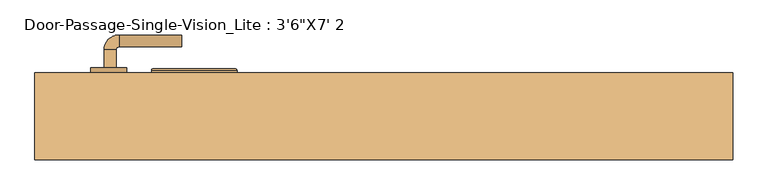
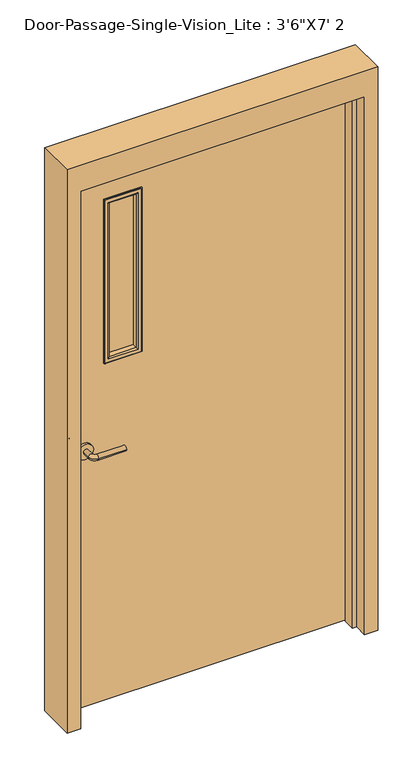
"""IFC4 building model written with IfcOpenShell, lengths in millimetres: door geometry."""

from ifc_helpers import new_model, si_unit, point, frame, frame_2d, origin, place, context, project, spatial, polyline, circle_curve, ellipse_curve, trimmed, segment, composite_curve, outline, extrude, faceted_brep, source, transform, mapped, element, save
from ifc_brep_helpers import plane_surface, cylinder_surface, revolved_surface, advanced_brep


def door_586e558e(model_context):
    return source(origin(), model_context, "Body", "SolidModel", [
        advanced_brep(
        [(-468.390625, 42.8, 1016.0), (-448.390625, 42.8, 1016.0), (-448.390625, 12.8, 1016.0), (-468.390625, 12.8, 1016.0), (-443.390625, 7.8, 1016.0), (-443.390625, -12.2, 1016.0), (-338.390625, -12.2, 1016.0), (-338.390625, 7.8, 1016.0)],
        [
            (0, 1, circle_curve(frame((-458.390625, 42.8, 1016.0), z_axis=(0.0, 1.0, 0.0), x_axis=(1.0, 0.0, 0.0)), 10.0)),
            (1, 0, circle_curve(frame((-458.390625, 42.8, 1016.0), z_axis=(0.0, 1.0, 0.0), x_axis=(1.0, 0.0, 0.0)), 10.0)),
            (1, 2),
            (2, 3, circle_curve(frame((-458.390625, 12.8, 1016.0), z_axis=(0.0, 1.0, 0.0), x_axis=(1.0, 0.0, 0.0)), 10.0)),
            (3, 0),
            (3, 2, circle_curve(frame((-458.390625, 12.8, 1016.0), z_axis=(0.0, 1.0, 0.0), x_axis=(1.0, 0.0, 0.0)), 10.0)),
            (4, 5, circle_curve(frame((-443.390625, -2.2, 1016.0), z_axis=(-1.0, 0.0, 0.0), x_axis=(0.0, 1.0, 0.0)), 10.0)),
            (5, 3, circle_curve(frame((-443.390625, 12.8, 1016.0), z_axis=(0.0, 0.0, -1.0), x_axis=(-1.0, 0.0, 0.0)), 25.0)),
            (2, 4, circle_curve(frame((-443.390625, 12.8, 1016.0), z_axis=(0.0, 0.0, 1.0), x_axis=(-1.0, 0.0, 0.0)), 5.0)),
            (5, 4, circle_curve(frame((-443.390625, -2.2, 1016.0), z_axis=(-1.0, 0.0, 0.0), x_axis=(0.0, 1.0, 0.0)), 10.0)),
            (6, 7, circle_curve(frame((-338.390625, -2.2, 1016.0), z_axis=(1.0, 0.0, 0.0), x_axis=(0.0, 1.0, 0.0)), 10.0)),
            (7, 6, circle_curve(frame((-338.390625, -2.2, 1016.0), z_axis=(1.0, 0.0, 0.0), x_axis=(0.0, 1.0, 0.0)), 10.0)),
            (4, 7),
            (6, 5),
        ],
        [
            plane_surface(frame((-458.390625, 42.8, 1016.0), z_axis=(0.0, 1.0, 0.0), x_axis=(0.0, 0.0, 1.0))),
            cylinder_surface(frame((-458.390625, 42.8, 1016.0), z_axis=(0.0, 1.0, 0.0), x_axis=(1.0, 0.0, 0.0)), 10.0),
            revolved_surface(trimmed(ellipse_curve(frame((-458.390625, 12.8, 1016.0), z_axis=(0.0, -1.0, 0.0), x_axis=(1.0, 0.0, 0.0)), 10.0, 10.0), [point((-468.390625, 12.8, 1016.0))], [point((-448.390625, 12.8, 1016.0))], True, "CARTESIAN"), (-443.390625, 12.8, 1016.0), (0.0, 0.0, -1.0)),
            revolved_surface(trimmed(ellipse_curve(frame((-458.390625, 12.8, 1016.0), z_axis=(0.0, -1.0, 0.0), x_axis=(1.0, 0.0, 0.0)), 10.0, 10.0), [point((-448.390625, 12.8, 1016.0))], [point((-468.390625, 12.8, 1016.0))], True, "CARTESIAN"), (-443.390625, 12.8, 1016.0), (0.0, 0.0, -1.0)),
            plane_surface(frame((-338.390625, -2.2, 1016.0), z_axis=(1.0, 0.0, 0.0), x_axis=(0.0, 0.0, 1.0))),
            cylinder_surface(frame((-443.390625, -2.2, 1016.0), z_axis=(-1.0, 0.0, 0.0), x_axis=(0.0, 1.0, 0.0)), 10.0),
        ],
        [
            (0, [[1, 2]]),
            (1, [[3, 4, 5, -2]]),
            (1, [[-5, 6, -3, -1]]),
            (2, [[7, 8, -4, 9]]),
            (3, [[10, -9, -6, -8]]),
            (4, [[11, 12]]),
            (5, [[13, -11, 14, -7]]),
            (5, [[-14, -12, -13, -10]]),
        ],
    ),
        extrude(outline(composite_curve([segment(trimmed(circle_curve(frame_2d((1016.0, -460.890625)), 30.0), [point((1016.0, -490.890625))], [point((1016.0, -430.890625))], False, "CARTESIAN"), True, "CONTINUOUS"), segment(trimmed(circle_curve(frame_2d((1016.0, -460.890625)), 30.0), [point((1016.0, -430.890625))], [point((1016.0, -490.890625))], False, "CARTESIAN"), True, "CONTINUOUS")], self_intersect=False)), frame((0.0, 42.8, 0.0), z_axis=(0.0, 1.0, 0.0), x_axis=(0.0, 0.0, 1.0)), (0.0, 0.0, 1.0), 8.0),
        advanced_brep(
        [(-468.390625, 103.25, 1016.0), (-448.390625, 103.25, 1016.0), (-468.390625, 133.25, 1016.0), (-448.390625, 133.25, 1016.0), (-443.390625, 138.25, 1016.0), (-443.390625, 158.25, 1016.0), (-338.390625, 158.25, 1016.0), (-338.390625, 138.25, 1016.0)],
        [
            (0, 1, circle_curve(frame((-458.390625, 103.25, 1016.0), z_axis=(0.0, -1.0, 0.0), x_axis=(1.0, 0.0, 0.0)), 10.0)),
            (1, 0, circle_curve(frame((-458.390625, 103.25, 1016.0), z_axis=(0.0, -1.0, 0.0), x_axis=(1.0, 0.0, 0.0)), 10.0)),
            (0, 2),
            (2, 3, circle_curve(frame((-458.390625, 133.25, 1016.0), z_axis=(0.0, -1.0, 0.0), x_axis=(1.0, 0.0, 0.0)), 10.0)),
            (3, 1),
            (3, 2, circle_curve(frame((-458.390625, 133.25, 1016.0), z_axis=(0.0, -1.0, 0.0), x_axis=(1.0, 0.0, 0.0)), 10.0)),
            (4, 3, circle_curve(frame((-443.390625, 133.25, 1016.0), z_axis=(0.0, 0.0, 1.0), x_axis=(-1.0, 0.0, 0.0)), 5.0)),
            (2, 5, circle_curve(frame((-443.390625, 133.25, 1016.0), z_axis=(0.0, 0.0, -1.0), x_axis=(-1.0, 0.0, 0.0)), 25.0)),
            (5, 4, circle_curve(frame((-443.390625, 148.25, 1016.0), z_axis=(-1.0, 0.0, 0.0), x_axis=(0.0, -1.0, 0.0)), 10.0)),
            (4, 5, circle_curve(frame((-443.390625, 148.25, 1016.0), z_axis=(-1.0, 0.0, 0.0), x_axis=(0.0, -1.0, 0.0)), 10.0)),
            (6, 7, circle_curve(frame((-338.390625, 148.25, 1016.0), z_axis=(1.0, 0.0, 0.0), x_axis=(0.0, -1.0, 0.0)), 10.0)),
            (7, 6, circle_curve(frame((-338.390625, 148.25, 1016.0), z_axis=(1.0, 0.0, 0.0), x_axis=(0.0, -1.0, 0.0)), 10.0)),
            (5, 6),
            (7, 4),
        ],
        [
            plane_surface(frame((-458.390625, 103.25, 1016.0), z_axis=(0.0, -1.0, 0.0), x_axis=(0.0, 0.0, 1.0))),
            cylinder_surface(frame((-458.390625, 103.25, 1016.0), z_axis=(0.0, -1.0, 0.0), x_axis=(1.0, 0.0, 0.0)), 10.0),
            revolved_surface(trimmed(ellipse_curve(frame((-458.390625, 133.25, 1016.0), z_axis=(0.0, -1.0, 0.0), x_axis=(1.0, 0.0, 0.0)), 10.0, 10.0), [point((-468.390625, 133.25, 1016.0))], [point((-448.390625, 133.25, 1016.0))], True, "CARTESIAN"), (-443.390625, 133.25, 1016.0), (0.0, 0.0, -1.0)),
            revolved_surface(trimmed(ellipse_curve(frame((-458.390625, 133.25, 1016.0), z_axis=(0.0, -1.0, 0.0), x_axis=(1.0, 0.0, 0.0)), 10.0, 10.0), [point((-448.390625, 133.25, 1016.0))], [point((-468.390625, 133.25, 1016.0))], True, "CARTESIAN"), (-443.390625, 133.25, 1016.0), (0.0, 0.0, -1.0)),
            plane_surface(frame((-338.390625, 148.25, 1016.0), z_axis=(1.0, 0.0, 0.0), x_axis=(0.0, 0.0, 1.0))),
            cylinder_surface(frame((-443.390625, 148.25, 1016.0), z_axis=(-1.0, 0.0, 0.0), x_axis=(0.0, -1.0, 0.0)), 10.0),
        ],
        [
            (0, [[1, 2]]),
            (1, [[-1, 3, 4, 5]]),
            (1, [[-2, -5, 6, -3]]),
            (2, [[7, -4, 8, 9]]),
            (3, [[-8, -6, -7, 10]]),
            (4, [[11, 12]]),
            (5, [[-9, 13, -12, 14]]),
            (5, [[-10, -14, -11, -13]]),
        ],
    ),
        extrude(outline(composite_curve([segment(trimmed(circle_curve(frame_2d((1016.0, -460.890625)), 30.0), [point((1016.0, -490.890625))], [point((1016.0, -430.890625))], False, "CARTESIAN"), True, "CONTINUOUS"), segment(trimmed(circle_curve(frame_2d((1016.0, -460.890625)), 30.0), [point((1016.0, -430.890625))], [point((1016.0, -490.890625))], False, "CARTESIAN"), True, "CONTINUOUS")], self_intersect=False)), frame((0.0, 95.25, 0.0), z_axis=(0.0, 1.0, 0.0), x_axis=(0.0, 0.0, 1.0)), (0.0, 0.0, 1.0), 8.0),
        extrude(outline(polyline([(2133.6, -533.4), (0.0, -533.4), (0.0, 533.4), (2133.6, 533.4), (2133.6, -533.4)]), holes=[polyline([(1981.2, -381.0), (1981.2, -254.0), (1346.2, -254.0), (1346.2, -381.0), (1981.2, -381.0)])]), frame((0.0, 50.8, 0.0), z_axis=(0.0, 1.0, 0.0), x_axis=(0.0, 0.0, 1.0)), (0.0, 0.0, 1.0), 44.45),
        faceted_brep([(533.4, 46.0375, 0.0), (533.4, 95.25, 0.0), (584.2, 95.25, 0.0), (584.2, -50.8, 0.0), (533.4, -50.8, 0.0), (533.4, -1.5875, 0.0), (517.525, -1.5875, 0.0), (517.525, 46.0375, 0.0), (533.4, 46.0375, 2133.6), (533.4, 95.25, 2133.6), (-533.4, 95.25, 2133.6), (-533.4, 95.25, 0.0), (-584.2, 95.25, 0.0), (-584.2, 95.25, 2235.2), (584.2, 95.25, 2235.2), (584.2, -50.8, 2235.2), (-584.2, -50.8, 2235.2), (-584.2, -50.8, 0.0), (-533.4, -50.8, 0.0), (-533.4, -50.8, 2133.6), (533.4, -50.8, 2133.6), (533.4, -1.5875, 2133.6), (-533.4, -1.5875, 2133.6), (-533.4, -1.5875, 0.0), (-517.525, -1.5875, 0.0), (-517.525, -1.5875, 2117.725), (517.525, -1.5875, 2117.725), (517.525, 46.0375, 2117.725), (-517.525, 46.0375, 2117.725), (-517.525, 46.0375, 0.0), (-533.4, 46.0375, 0.0), (-533.4, 46.0375, 2133.6)], [[[0, 1, 2, 3, 4, 5, 6, 7]], [[1, 0, 8, 9]], [[2, 1, 9, 10, 11, 12, 13, 14]], [[3, 2, 14, 15]], [[4, 3, 15, 16, 17, 18, 19, 20]], [[5, 4, 20, 21]], [[6, 5, 21, 22, 23, 24, 25, 26]], [[7, 6, 26, 27]], [[0, 7, 27, 28, 29, 30, 31, 8]], [[9, 8, 31, 10]], [[20, 19, 22, 21]], [[26, 25, 28, 27]], [[12, 11, 30, 29, 24, 23, 18, 17]], [[11, 10, 31, 30]], [[13, 12, 17, 16]], [[19, 18, 23, 22]], [[25, 24, 29, 28]], [[15, 14, 13, 16]]]),
        extrude(outline(polyline([(-254.0, 69.85), (-381.0, 69.85), (-381.0, 76.2), (-254.0, 76.2), (-254.0, 69.85)])), frame((0.0, 0.0, 1346.2), z_axis=(0.0, 0.0, 1.0), x_axis=(1.0, 0.0, 0.0)), (0.0, 0.0, 1.0), 635.0),
        advanced_brep(
        [(-381.0, 76.2, 1981.2), (-381.0, 95.25, 1981.2), (-381.0, 95.25, 1346.2), (-381.0, 76.2, 1346.2), (-369.0, 96.25, 1969.2), (-369.0, 76.2, 1969.2), (-369.0, 76.2, 1358.2), (-369.0, 96.25, 1358.2), (-374.0, 101.25, 1974.2), (-374.0, 101.25, 1353.2), (-389.0, 99.25, 1989.2), (-387.0, 101.25, 1987.2), (-387.0, 101.25, 1340.2), (-389.0, 99.25, 1338.2), (-389.0, 95.25, 1989.2), (-389.0, 95.25, 1338.2), (-254.0, 95.25, 1346.2), (-254.0, 76.2, 1346.2), (-266.0, 76.2, 1358.2), (-266.0, 96.25, 1358.2), (-261.0, 101.25, 1353.2), (-248.0, 101.25, 1340.2), (-246.0, 99.25, 1338.2), (-246.0, 95.25, 1338.2), (-254.0, 95.25, 1981.2), (-254.0, 76.2, 1981.2), (-266.0, 76.2, 1969.2), (-266.0, 96.25, 1969.2), (-261.0, 101.25, 1974.2), (-248.0, 101.25, 1987.2), (-246.0, 99.25, 1989.2), (-246.0, 95.25, 1989.2)],
        [
            (0, 1),
            (1, 2),
            (2, 3),
            (3, 0),
            (4, 5),
            (5, 6),
            (6, 7),
            (7, 4),
            (8, 4, ellipse_curve(frame((-374.0, 96.25, 1974.2), z_axis=(-0.7071067811865475, 0.0, -0.7071067811865475), x_axis=(-0.7071067811865474, 0.0, 0.7071067811865476)), 7.0710678, 5.0)),
            (7, 9, ellipse_curve(frame((-374.0, 96.25, 1353.2), z_axis=(-0.7071067811865475, 0.0, 0.7071067811865475), x_axis=(0.7071067811865474, 0.0, 0.7071067811865476)), 7.0710678, 5.0)),
            (9, 8),
            (10, 11, ellipse_curve(frame((-387.0, 99.25, 1987.2), z_axis=(-0.7071067811865475, 0.0, -0.7071067811865475), x_axis=(-0.7071067811865474, 0.0, 0.7071067811865476)), 2.8284271, 2.0)),
            (11, 12),
            (12, 13, ellipse_curve(frame((-387.0, 99.25, 1340.2), z_axis=(-0.7071067811865475, 0.0, 0.7071067811865475), x_axis=(0.7071067811865474, 0.0, 0.7071067811865476)), 2.8284271, 2.0)),
            (13, 10),
            (14, 10),
            (13, 15),
            (15, 14),
            (2, 16),
            (16, 17),
            (17, 3),
            (6, 18),
            (18, 19),
            (19, 7),
            (19, 20, ellipse_curve(frame((-261.0, 96.25, 1353.2), z_axis=(-0.7071067811865475, 0.0, -0.7071067811865475), x_axis=(-0.7071067811865476, 0.0, 0.7071067811865474)), 7.0710678, 5.0)),
            (20, 9),
            (12, 21),
            (21, 22, ellipse_curve(frame((-248.0, 99.25, 1340.2), z_axis=(-0.7071067811865475, 0.0, -0.7071067811865475), x_axis=(-0.7071067811865476, 0.0, 0.7071067811865474)), 2.8284271, 2.0)),
            (22, 13),
            (22, 23),
            (23, 15),
            (16, 24),
            (24, 25),
            (25, 17),
            (18, 26),
            (26, 27),
            (27, 19),
            (27, 28, ellipse_curve(frame((-261.0, 96.25, 1974.2), z_axis=(0.7071067811865475, 0.0, -0.7071067811865475), x_axis=(-0.7071067811865474, 0.0, -0.7071067811865476)), 7.0710678, 5.0)),
            (28, 20),
            (21, 29),
            (29, 30, ellipse_curve(frame((-248.0, 99.25, 1987.2), z_axis=(0.7071067811865475, 0.0, -0.7071067811865475), x_axis=(-0.7071067811865474, 0.0, -0.7071067811865476)), 2.8284271, 2.0)),
            (30, 22),
            (30, 31),
            (31, 23),
            (31, 14),
            (1, 24),
            (0, 25),
            (5, 26),
            (4, 27),
            (8, 28),
            (11, 29),
            (10, 30),
        ],
        [
            plane_surface(frame((-381.0, 95.25, 1981.2), z_axis=(-1.0, 0.0, 0.0), x_axis=(0.0, 0.0, -1.0))),
            plane_surface(frame((-369.0, 76.2, 1969.2), z_axis=(1.0, 0.0, 0.0), x_axis=(0.0, 0.0, -1.0))),
            cylinder_surface(frame((-374.0, 96.25, 1981.2), z_axis=(0.0, 0.0, 1.0), x_axis=(-1.0, 0.0, 0.0)), 5.0),
            cylinder_surface(frame((-387.0, 99.25, 1981.2), z_axis=(0.0, 0.0, 1.0), x_axis=(-1.0, 0.0, 0.0)), 2.0),
            plane_surface(frame((-389.0, 99.25, 1989.2), z_axis=(-1.0, 0.0, 0.0), x_axis=(0.0, 0.0, -1.0))),
            plane_surface(frame((-381.0, 95.25, 1346.2), z_axis=(0.0, 0.0, -1.0), x_axis=(1.0, 0.0, 0.0))),
            plane_surface(frame((-369.0, 76.2, 1358.2), z_axis=(0.0, 0.0, 1.0), x_axis=(1.0, 0.0, 0.0))),
            cylinder_surface(frame((-381.0, 96.25, 1353.2), z_axis=(-1.0, 0.0, 0.0), x_axis=(0.0, 0.0, -1.0)), 5.0),
            cylinder_surface(frame((-381.0, 99.25, 1340.2), z_axis=(-1.0, 0.0, 0.0), x_axis=(0.0, 0.0, -1.0)), 2.0),
            plane_surface(frame((-389.0, 99.25, 1338.2), z_axis=(0.0, 0.0, -1.0), x_axis=(1.0, 0.0, 0.0))),
            plane_surface(frame((-254.0, 95.25, 1346.2), z_axis=(1.0, 0.0, 0.0), x_axis=(0.0, 0.0, 1.0))),
            plane_surface(frame((-266.0, 76.2, 1358.2), z_axis=(-1.0, 0.0, 0.0), x_axis=(0.0, 0.0, 1.0))),
            cylinder_surface(frame((-261.0, 96.25, 1346.2), z_axis=(0.0, 0.0, -1.0), x_axis=(1.0, 0.0, 0.0)), 5.0),
            cylinder_surface(frame((-248.0, 99.25, 1346.2), z_axis=(0.0, 0.0, -1.0), x_axis=(1.0, 0.0, 0.0)), 2.0),
            plane_surface(frame((-246.0, 99.25, 1338.2), z_axis=(1.0, 0.0, 0.0), x_axis=(0.0, 0.0, 1.0))),
            plane_surface(frame((-246.0, 95.25, 1989.2), z_axis=(0.0, -1.0, 0.0), x_axis=(-1.0, 0.0, 0.0))),
            plane_surface(frame((-254.0, 95.25, 1981.2), z_axis=(0.0, 0.0, 1.0), x_axis=(-1.0, 0.0, 0.0))),
            plane_surface(frame((-254.0, 76.2, 1981.2), z_axis=(0.0, -1.0, 0.0), x_axis=(-1.0, 0.0, 0.0))),
            plane_surface(frame((-266.0, 76.2, 1969.2), z_axis=(0.0, 0.0, -1.0), x_axis=(-1.0, 0.0, 0.0))),
            cylinder_surface(frame((-254.0, 96.25, 1974.2), z_axis=(1.0, 0.0, 0.0), x_axis=(0.0, 0.0, 1.0)), 5.0),
            plane_surface(frame((-261.0, 101.25, 1974.2), z_axis=(0.0, 1.0, 0.0), x_axis=(-1.0, 0.0, 0.0))),
            cylinder_surface(frame((-254.0, 99.25, 1987.2), z_axis=(1.0, 0.0, 0.0), x_axis=(0.0, 0.0, 1.0)), 2.0),
            plane_surface(frame((-246.0, 99.25, 1989.2), z_axis=(0.0, 0.0, 1.0), x_axis=(-1.0, 0.0, 0.0))),
        ],
        [
            (0, [[1, 2, 3, 4]]),
            (1, [[5, 6, 7, 8]]),
            (2, [[9, -8, 10, 11]]),
            (3, [[12, 13, 14, 15]]),
            (4, [[16, -15, 17, 18]]),
            (5, [[-3, 19, 20, 21]]),
            (6, [[-7, 22, 23, 24]]),
            (7, [[-10, -24, 25, 26]]),
            (8, [[-14, 27, 28, 29]]),
            (9, [[-17, -29, 30, 31]]),
            (10, [[-20, 32, 33, 34]]),
            (11, [[-23, 35, 36, 37]]),
            (12, [[-25, -37, 38, 39]]),
            (13, [[-28, 40, 41, 42]]),
            (14, [[-30, -42, 43, 44]]),
            (15, [[-31, -44, 45, -18], [46, -32, -19, -2]]),
            (16, [[-33, -46, -1, 47]]),
            (17, [[-21, -34, -47, -4], [48, -35, -22, -6]]),
            (18, [[-36, -48, -5, 49]]),
            (19, [[-38, -49, -9, 50]]),
            (20, [[51, -40, -27, -13], [-26, -39, -50, -11]]),
            (21, [[-41, -51, -12, 52]]),
            (22, [[-43, -52, -16, -45]]),
        ],
    ),
        advanced_brep(
        [(-381.0, 69.85, 1346.2), (-381.0, 50.8, 1346.2), (-381.0, 50.8, 1981.2), (-381.0, 69.85, 1981.2), (-369.0, 49.8, 1358.2), (-369.0, 69.85, 1358.2), (-369.0, 69.85, 1969.2), (-369.0, 49.8, 1969.2), (-374.0, 44.8, 1353.2), (-374.0, 44.8, 1974.2), (-389.0, 46.8, 1338.2), (-387.0, 44.8, 1340.2), (-387.0, 44.8, 1987.2), (-389.0, 46.8, 1989.2), (-389.0, 50.8, 1338.2), (-389.0, 50.8, 1989.2), (-254.0, 50.8, 1981.2), (-254.0, 69.85, 1981.2), (-266.0, 69.85, 1969.2), (-266.0, 49.8, 1969.2), (-261.0, 44.8, 1974.2), (-248.0, 44.8, 1987.2), (-246.0, 46.8, 1989.2), (-246.0, 50.8, 1989.2), (-254.0, 50.8, 1346.2), (-254.0, 69.85, 1346.2), (-266.0, 69.85, 1358.2), (-266.0, 49.8, 1358.2), (-261.0, 44.8, 1353.2), (-248.0, 44.8, 1340.2), (-246.0, 46.8, 1338.2), (-246.0, 50.8, 1338.2)],
        [
            (0, 1),
            (1, 2),
            (2, 3),
            (3, 0),
            (4, 5),
            (5, 6),
            (6, 7),
            (7, 4),
            (8, 4, ellipse_curve(frame((-374.0, 49.8, 1353.2), z_axis=(-0.7071067811865475, 0.0, 0.7071067811865475), x_axis=(-0.7071067811865474, 0.0, -0.7071067811865476)), 7.0710678, 5.0)),
            (7, 9, ellipse_curve(frame((-374.0, 49.8, 1974.2), z_axis=(-0.7071067811865475, 0.0, -0.7071067811865475), x_axis=(0.7071067811865474, 0.0, -0.7071067811865476)), 7.0710678, 5.0)),
            (9, 8),
            (10, 11, ellipse_curve(frame((-387.0, 46.8, 1340.2), z_axis=(-0.7071067811865475, 0.0, 0.7071067811865475), x_axis=(-0.7071067811865474, 0.0, -0.7071067811865476)), 2.8284271, 2.0)),
            (11, 12),
            (12, 13, ellipse_curve(frame((-387.0, 46.8, 1987.2), z_axis=(-0.7071067811865475, 0.0, -0.7071067811865475), x_axis=(0.7071067811865474, 0.0, -0.7071067811865476)), 2.8284271, 2.0)),
            (13, 10),
            (14, 10),
            (13, 15),
            (15, 14),
            (2, 16),
            (16, 17),
            (17, 3),
            (6, 18),
            (18, 19),
            (19, 7),
            (19, 20, ellipse_curve(frame((-261.0, 49.8, 1974.2), z_axis=(-0.7071067811865475, 0.0, 0.7071067811865475), x_axis=(-0.7071067811865476, 0.0, -0.7071067811865474)), 7.0710678, 5.0)),
            (20, 9),
            (12, 21),
            (21, 22, ellipse_curve(frame((-248.0, 46.8, 1987.2), z_axis=(-0.7071067811865475, 0.0, 0.7071067811865475), x_axis=(-0.7071067811865476, 0.0, -0.7071067811865474)), 2.8284271, 2.0)),
            (22, 13),
            (22, 23),
            (23, 15),
            (16, 24),
            (24, 25),
            (25, 17),
            (18, 26),
            (26, 27),
            (27, 19),
            (27, 28, ellipse_curve(frame((-261.0, 49.8, 1353.2), z_axis=(0.7071067811865475, 0.0, 0.7071067811865475), x_axis=(-0.7071067811865474, 0.0, 0.7071067811865476)), 7.0710678, 5.0)),
            (28, 20),
            (21, 29),
            (29, 30, ellipse_curve(frame((-248.0, 46.8, 1340.2), z_axis=(0.7071067811865475, 0.0, 0.7071067811865475), x_axis=(-0.7071067811865474, 0.0, 0.7071067811865476)), 2.8284271, 2.0)),
            (30, 22),
            (30, 31),
            (31, 23),
            (31, 14),
            (1, 24),
            (0, 25),
            (5, 26),
            (4, 27),
            (8, 28),
            (11, 29),
            (10, 30),
        ],
        [
            plane_surface(frame((-381.0, 50.8, 1346.2), z_axis=(-1.0, 0.0, 0.0), x_axis=(0.0, 0.0, 1.0))),
            plane_surface(frame((-369.0, 69.85, 1358.2), z_axis=(1.0, 0.0, 0.0), x_axis=(0.0, 0.0, 1.0))),
            cylinder_surface(frame((-374.0, 49.8, 1346.2), z_axis=(0.0, 0.0, -1.0), x_axis=(-1.0, 0.0, 0.0)), 5.0),
            cylinder_surface(frame((-387.0, 46.8, 1346.2), z_axis=(0.0, 0.0, -1.0), x_axis=(-1.0, 0.0, 0.0)), 2.0),
            plane_surface(frame((-389.0, 46.8, 1338.2), z_axis=(-1.0, 0.0, 0.0), x_axis=(0.0, 0.0, 1.0))),
            plane_surface(frame((-381.0, 50.8, 1981.2), z_axis=(0.0, 0.0, 1.0), x_axis=(1.0, 0.0, 0.0))),
            plane_surface(frame((-369.0, 69.85, 1969.2), z_axis=(0.0, 0.0, -1.0), x_axis=(1.0, 0.0, 0.0))),
            cylinder_surface(frame((-381.0, 49.8, 1974.2), z_axis=(-1.0, 0.0, 0.0), x_axis=(0.0, 0.0, 1.0)), 5.0),
            cylinder_surface(frame((-381.0, 46.8, 1987.2), z_axis=(-1.0, 0.0, 0.0), x_axis=(0.0, 0.0, 1.0)), 2.0),
            plane_surface(frame((-389.0, 46.8, 1989.2), z_axis=(0.0, 0.0, 1.0), x_axis=(1.0, 0.0, 0.0))),
            plane_surface(frame((-254.0, 50.8, 1981.2), z_axis=(1.0, 0.0, 0.0), x_axis=(0.0, 0.0, -1.0))),
            plane_surface(frame((-266.0, 69.85, 1969.2), z_axis=(-1.0, 0.0, 0.0), x_axis=(0.0, 0.0, -1.0))),
            cylinder_surface(frame((-261.0, 49.8, 1981.2), z_axis=(0.0, 0.0, 1.0), x_axis=(1.0, 0.0, 0.0)), 5.0),
            cylinder_surface(frame((-248.0, 46.8, 1981.2), z_axis=(0.0, 0.0, 1.0), x_axis=(1.0, 0.0, 0.0)), 2.0),
            plane_surface(frame((-246.0, 46.8, 1989.2), z_axis=(1.0, 0.0, 0.0), x_axis=(0.0, 0.0, -1.0))),
            plane_surface(frame((-246.0, 50.8, 1338.2), z_axis=(0.0, 1.0, 0.0), x_axis=(-1.0, 0.0, 0.0))),
            plane_surface(frame((-254.0, 50.8, 1346.2), z_axis=(0.0, 0.0, -1.0), x_axis=(-1.0, 0.0, 0.0))),
            plane_surface(frame((-254.0, 69.85, 1346.2), z_axis=(0.0, 1.0, 0.0), x_axis=(-1.0, 0.0, 0.0))),
            plane_surface(frame((-266.0, 69.85, 1358.2), z_axis=(0.0, 0.0, 1.0), x_axis=(-1.0, 0.0, 0.0))),
            cylinder_surface(frame((-254.0, 49.8, 1353.2), z_axis=(1.0, 0.0, 0.0), x_axis=(0.0, 0.0, -1.0)), 5.0),
            plane_surface(frame((-261.0, 44.8, 1353.2), z_axis=(0.0, -1.0, 0.0), x_axis=(-1.0, 0.0, 0.0))),
            cylinder_surface(frame((-254.0, 46.8, 1340.2), z_axis=(1.0, 0.0, 0.0), x_axis=(0.0, 0.0, -1.0)), 2.0),
            plane_surface(frame((-246.0, 46.8, 1338.2), z_axis=(0.0, 0.0, -1.0), x_axis=(-1.0, 0.0, 0.0))),
        ],
        [
            (0, [[1, 2, 3, 4]]),
            (1, [[5, 6, 7, 8]]),
            (2, [[9, -8, 10, 11]]),
            (3, [[12, 13, 14, 15]]),
            (4, [[16, -15, 17, 18]]),
            (5, [[-3, 19, 20, 21]]),
            (6, [[-7, 22, 23, 24]]),
            (7, [[-10, -24, 25, 26]]),
            (8, [[-14, 27, 28, 29]]),
            (9, [[-17, -29, 30, 31]]),
            (10, [[-20, 32, 33, 34]]),
            (11, [[-23, 35, 36, 37]]),
            (12, [[-25, -37, 38, 39]]),
            (13, [[-28, 40, 41, 42]]),
            (14, [[-30, -42, 43, 44]]),
            (15, [[-31, -44, 45, -18], [46, -32, -19, -2]]),
            (16, [[-33, -46, -1, 47]]),
            (17, [[-21, -34, -47, -4], [48, -35, -22, -6]]),
            (18, [[-36, -48, -5, 49]]),
            (19, [[-38, -49, -9, 50]]),
            (20, [[51, -40, -27, -13], [-26, -39, -50, -11]]),
            (21, [[-41, -51, -12, 52]]),
            (22, [[-43, -52, -16, -45]]),
        ],
    ),
    ])


if __name__ == "__main__":
    model = new_model("IFC4")
    model_context = context("Model", 3, world=origin())
    ifc_project = project(units=[si_unit("LENGTHUNIT", "METRE", prefix="MILLI")], contexts=[model_context])
    site = spatial("IfcSite", under=ifc_project)
    building = spatial("IfcBuilding", under=site)
    placement = place(None, origin())
    door_shape = door_586e558e(model_context)
    element("IfcDoor", 1, ObjectType="Door-Passage-Single-Vision_Lite : 3'6\"X7' 2", at=placement, inside=building, context=model_context, shape_type="MappedRepresentation", body=[
        mapped(door_shape, transform((0.0, 0.0, 0.0), x_axis=(1.0, 0.0, 0.0), y_axis=(0.0, 1.0, 0.0), z_axis=(0.0, 0.0, 1.0))),
    ])
    save(model, "model.ifc")

# Revit data of these elements
# Type "Door-Passage-Single-Vision_Lite : 3'6\"X7' 2"
#   Type Mark = "14"
#   Assembly Code = "B2030100"
#   Analytic Construction = "Wooden"
#   Thickness = 0' - 1 3/4"
#   Thermal Resistance (R) = 2.5876 (h·ft²·°F)/BTU
#   Swing Angle [instance default] = 90.00°
#   Strike Height = 3' - 4"
#   Rough Width [instance default] = 3' - 10"
#   Rough Height [instance default] = 7' - 4"
#   MFOpeningHeight [instance default] = 0' - 4"
#   MFOpeningWidth [instance default] = 0' - 4"
#   Inset Calculate [instance default] = 0' - 4"
#   Masonry Inset [instance default] = 0' - 1"
#   Height = 7' - 0"
#   Width = 3' - 6"
#   Heat Transfer Coefficient (U) = 0.3865 BTU/(h·ft²·°F)
#   Masonry Frame Depth = 0' - 5 3/4"
#   Masonry Frame [instance default] = yes
#   Function = 1
#   Dry Wall Frame [instance default] = no
#   Panel Material = Wood - Birch
#   Glazing = Glass
#   Glass Stop Material = Metal - Paint Finish - Grey
#   Frame Material = Metal - Paint Finish - Grey
#   Door Handle Material = Aluminum
#   Visual Light Transmittance = 0
#   Solar Heat Gain Coefficient = 0
#   Wall Closure = (empty or 0)
# Element 1 (IfcDoor, "Door-Passage-Single-Vision_Lite : 3'6\"X7' 2")
#   Materials on its faces: "Metal - Paint Finish - Grey", "Aluminum", "Wood - Birch", "Glass"
# Materials
#   "Wood - Birch": class "Wood", colour RGB 166 116 52, transparency 0, Cost = 0
#   "Glass": class "Glass", colour RGB 0 128 192, transparency 0.75, Description = "Soda Lime Glass", Cost = 0
#   "Metal - Paint Finish - Grey": class "Paint", colour RGB 104 104 104, transparency 0, Cost = 0
#   "Aluminum": class "Metal", colour RGB 247 247 247, transparency 0, Description = "Aluminum 6061", Cost = 0
